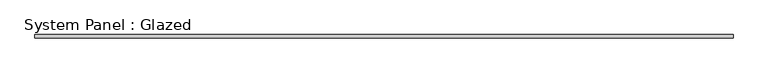
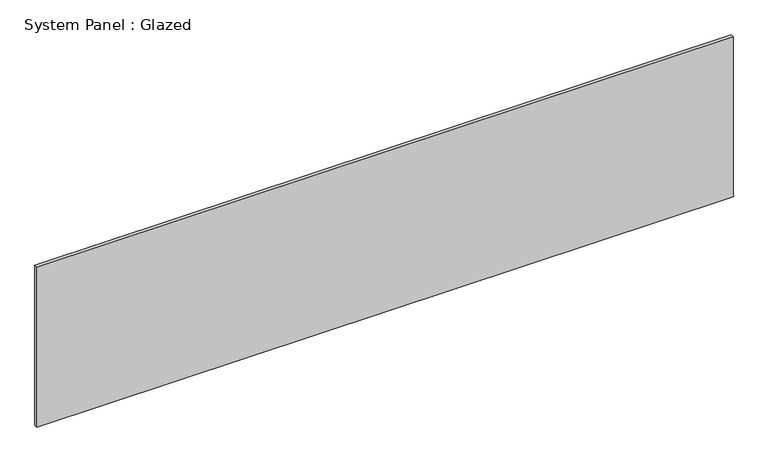
"""IFC4 building model written with IfcOpenShell, lengths in millimetres: plate geometry, System Panel : Glazed."""

from ifc_helpers import new_model, si_unit, origin, origin_with_axes, place, context, project, spatial, polyline, outline, extrude, source, transform, mapped, element, save


def system_panel_glazed_48506e1c(model_context):
    return source(origin(), model_context, "Body", "SweptSolid", [
        extrude(outline(polyline([(2514.6, -44.45), (-2514.6, -44.45), (-2514.6, -19.05), (2514.6, -19.05), (2514.6, -44.45)])), origin_with_axes(), (0.0, 0.0, 1.0), 1219.2),
    ])


if __name__ == "__main__":
    model = new_model("IFC4")
    model_context = context("Model", 3, world=origin())
    ifc_project = project(units=[si_unit("LENGTHUNIT", "METRE", prefix="MILLI")], contexts=[model_context])
    site = spatial("IfcSite", under=ifc_project)
    building = spatial("IfcBuilding", under=site)
    placement = place(None, origin())
    system_panel_glazed_shape = system_panel_glazed_48506e1c(model_context)
    element("IfcPlate", 1, ObjectType="System Panel : Glazed", at=placement, inside=building, context=model_context, shape_type="MappedRepresentation", body=[
        mapped(system_panel_glazed_shape, transform((0.0, 0.0, 0.0), x_axis=(1.0, 0.0, 0.0), y_axis=(0.0, 1.0, 0.0), z_axis=(0.0, 0.0, 1.0))),
    ])
    save(model, "model.ifc")

# Revit data of these elements
# Type "System Panel : Glazed"
#   Construction Type Id = "GSP4R"
#   Analytic Construction = "1/8 in Pilkington single glazing"
#   Visual Light Transmittance = 0.9
#   Solar Heat Gain Coefficient = 0.86
#   Heat Transfer Coefficient (U) = 1.18115 BTU/(h·ft²·°F)
# Element 1 (IfcPlate, "System Panel : Glazed")
#   Materials on its faces: "Glass"
# Materials
#   "Glass": class "Glass", colour RGB 0 128 192, transparency 0.75, Description = "Soda Lime Glass", Cost = 0
